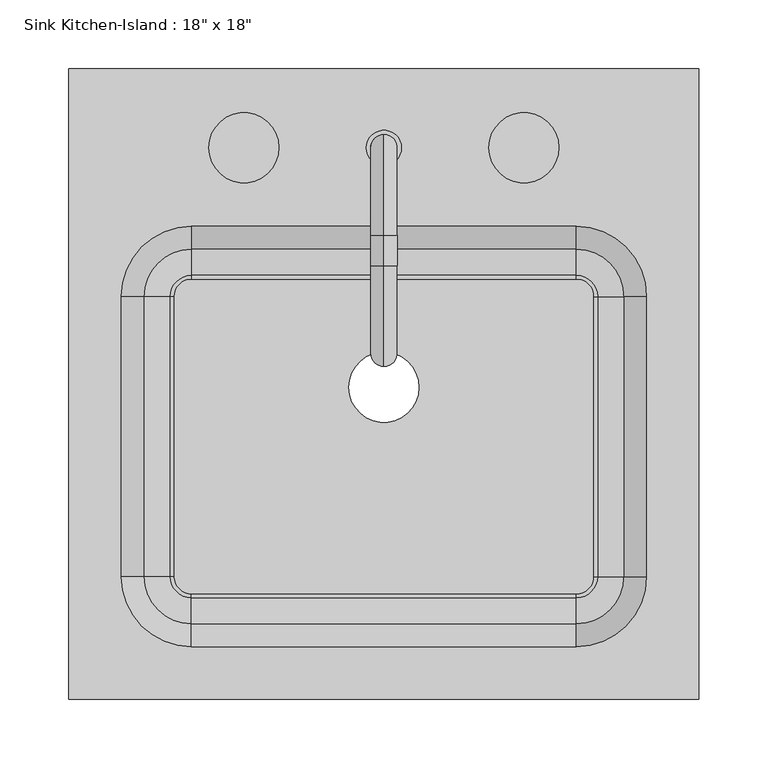
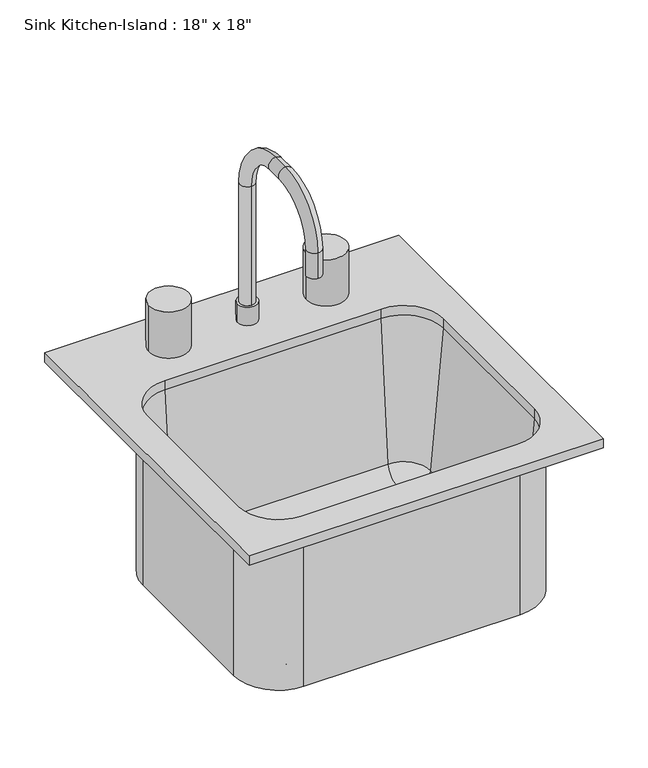
"""IFC4 building model written with IfcOpenShell, lengths in millimetres: flow terminal geometry."""

from ifc_helpers import new_model, si_unit, point, frame, frame_2d, origin, place, context, project, spatial, polyline, circle_curve, ellipse_curve, trimmed, segment, composite_curve, outline, extrude, source, transform, mapped, element, save
from ifc_brep_helpers import plane_surface, cylinder_surface, revolved_surface, advanced_brep


def flow_terminal_871c2e40(model_context):
    return source(origin(), model_context, "Body", "SolidModel", [
        advanced_brep(
        [(244.2892406, 230.9454011, 927.1), (-212.9107594, 230.9454011, 927.1), (-212.9107594, -226.2545989, 927.1), (244.2892406, -226.2545989, 927.1), (155.3892406, 116.6454011, 927.1), (206.1892406, 65.8454011, 927.1), (206.1892406, -137.3545989, 927.1), (155.3892406, -188.1545989, 927.1), (-124.0107594, -188.1545989, 927.1), (-174.8107594, -137.3545989, 927.1), (-174.8107594, 65.8454011, 927.1), (-124.0107594, 116.6454011, 927.1), (244.2892406, 230.9454011, 914.4), (244.2892406, -226.2545989, 914.4), (-212.9107594, -226.2545989, 914.4), (-212.9107594, 230.9454011, 914.4), (212.5392406, 65.8454011, 914.4), (155.3892406, 122.9954011, 914.4), (-124.0107594, 122.9954011, 914.4), (-181.1607594, 65.8454011, 914.4), (-181.1607594, -137.3545989, 914.4), (-124.0107594, -194.5045989, 914.4), (155.3892406, -194.5045989, 914.4), (212.5392406, -137.3545989, 914.4), (155.3892406, 116.6454011, 914.4), (206.1892406, 65.8454011, 914.4), (206.1892406, -137.3545989, 914.4), (155.3892406, -188.1545989, 914.4), (-124.0107594, -188.1545989, 914.4), (-174.8107594, -137.3545989, 914.4), (-174.8107594, 65.8454011, 914.4), (-124.0107594, 116.6454011, 914.4), (212.5392406, 65.8454011, 698.5), (155.3892406, 122.9954011, 698.5), (168.0892406, 65.8454011, 698.5), (155.3892406, 78.5454011, 698.5), (168.0892406, 65.8454011, 708.025), (155.3892406, 78.5454011, 708.025), (170.6776588, 65.8454011, 708.025), (155.3892406, 81.1338193, 708.025), (189.6551678, 65.8454011, 725.4146831), (155.3892406, 100.1113283, 725.4146831), (212.5392406, -137.3545989, 698.5), (168.0892406, -137.3545989, 698.5), (168.0892406, -137.3545989, 708.025), (170.6776588, -137.3545989, 708.025), (189.6551678, -137.3545989, 725.4146831), (155.3892406, -194.5045989, 698.5), (155.3892406, -150.0545989, 698.5), (155.3892406, -150.0545989, 708.025), (155.3892406, -152.6430171, 708.025), (155.3892406, -171.6205261, 725.4146831), (-124.0107594, -194.5045989, 698.5), (-124.0107594, -150.0545989, 698.5), (-124.0107594, -150.0545989, 708.025), (-124.0107594, -152.6430171, 708.025), (-124.0107594, -171.6205261, 725.4146831), (-181.1607594, -137.3545989, 698.5), (-136.7107594, -137.3545989, 698.5), (-136.7107594, -137.3545989, 708.025), (-139.2991776, -137.3545989, 708.025), (-158.2766866, -137.3545989, 725.4146831), (-181.1607594, 65.8454011, 698.5), (-136.7107594, 65.8454011, 698.5), (-136.7107594, 65.8454011, 708.025), (-139.2991776, 65.8454011, 708.025), (-158.2766866, 65.8454011, 725.4146831), (-124.0107594, 122.9954011, 698.5), (-124.0107594, 78.5454011, 698.5), (-124.0107594, 78.5454011, 708.025), (-124.0107594, 81.1338193, 708.025), (-124.0107594, 100.1113283, 725.4146831)],
        [
            (0, 1),
            (1, 2),
            (2, 3),
            (3, 0),
            (4, 5, circle_curve(frame((155.3892406, 65.8454011, 927.1), z_axis=(0.0, 0.0, -1.0), x_axis=(1.0, 0.0, 0.0)), 50.8)),
            (5, 6),
            (6, 7, circle_curve(frame((155.3892406, -137.3545989, 927.1), z_axis=(0.0, 0.0, -1.0), x_axis=(1.0, 0.0, 0.0)), 50.8)),
            (7, 8),
            (8, 9, circle_curve(frame((-124.0107594, -137.3545989, 927.1), z_axis=(0.0, 0.0, -1.0), x_axis=(1.0, 0.0, 0.0)), 50.8)),
            (9, 10),
            (10, 11, circle_curve(frame((-124.0107594, 65.8454011, 927.1), z_axis=(0.0, 0.0, -1.0), x_axis=(1.0, 0.0, 0.0)), 50.8)),
            (11, 4),
            (12, 13),
            (13, 14),
            (14, 15),
            (15, 12),
            (16, 17, circle_curve(frame((155.3892406, 65.8454011, 914.4), z_axis=(0.0, 0.0, 1.0), x_axis=(0.0, 1.0, 0.0)), 57.15)),
            (17, 18),
            (18, 19, circle_curve(frame((-124.0107594, 65.8454011, 914.4), z_axis=(0.0, 0.0, 1.0), x_axis=(-1.0, 0.0, 0.0)), 57.15)),
            (19, 20),
            (20, 21, circle_curve(frame((-124.0107594, -137.3545989, 914.4), z_axis=(0.0, 0.0, 1.0), x_axis=(0.0, -1.0, 0.0)), 57.15)),
            (21, 22),
            (22, 23, circle_curve(frame((155.3892406, -137.3545989, 914.4), z_axis=(0.0, 0.0, 1.0), x_axis=(1.0, 0.0, 0.0)), 57.15)),
            (23, 16),
            (0, 12),
            (15, 1),
            (14, 2),
            (13, 3),
            (4, 24),
            (24, 25, circle_curve(frame((155.3892406, 65.8454011, 914.4), z_axis=(0.0, 0.0, -1.0), x_axis=(1.0, 0.0, 0.0)), 50.8)),
            (25, 5),
            (25, 26),
            (26, 6),
            (26, 27, circle_curve(frame((155.3892406, -137.3545989, 914.4), z_axis=(0.0, 0.0, -1.0), x_axis=(1.0, 0.0, 0.0)), 50.8)),
            (27, 7),
            (27, 28),
            (28, 8),
            (28, 29, circle_curve(frame((-124.0107594, -137.3545989, 914.4), z_axis=(0.0, 0.0, -1.0), x_axis=(1.0, 0.0, 0.0)), 50.8)),
            (29, 9),
            (29, 30),
            (30, 10),
            (30, 31, circle_curve(frame((-124.0107594, 65.8454011, 914.4), z_axis=(0.0, 0.0, -1.0), x_axis=(1.0, 0.0, 0.0)), 50.8)),
            (31, 11),
            (31, 24),
            (32, 33, circle_curve(frame((155.3892406, 65.8454011, 698.5), z_axis=(0.0, 0.0, 1.0), x_axis=(0.0, 1.0, 0.0)), 57.15)),
            (33, 17),
            (16, 32),
            (32, 34),
            (34, 35, circle_curve(frame((155.3892406, 65.8454011, 698.5), z_axis=(0.0, 0.0, 1.0), x_axis=(0.0, 1.0, 0.0)), 12.7)),
            (35, 33),
            (34, 36),
            (36, 37, circle_curve(frame((155.3892406, 65.8454011, 708.025), z_axis=(0.0, 0.0, 1.0), x_axis=(0.0, 1.0, 0.0)), 12.7)),
            (37, 35),
            (36, 38),
            (38, 39, circle_curve(frame((155.3892406, 65.8454011, 708.025), z_axis=(0.0, 0.0, 1.0), x_axis=(0.0, 1.0, 0.0)), 15.2884182)),
            (39, 37),
            (38, 40, circle_curve(frame((170.6776588, 65.8454011, 727.075), z_axis=(0.0, -1.0, 0.0), x_axis=(1.0, 0.0, 0.0)), 19.05)),
            (40, 41, circle_curve(frame((155.3892406, 65.8454011, 725.4146831), z_axis=(0.0, 0.0, 1.0), x_axis=(0.0, 1.0, 0.0)), 34.2659272)),
            (41, 39, circle_curve(frame((155.3892406, 81.1338193, 727.075), z_axis=(-1.0, 0.0, 0.0), x_axis=(0.0, 1.0, 0.0)), 19.05)),
            (40, 25),
            (24, 41),
            (23, 42),
            (42, 32),
            (42, 43),
            (43, 34),
            (43, 44),
            (44, 36),
            (44, 45),
            (45, 38),
            (45, 46, circle_curve(frame((170.6776588, -137.3545989, 727.075), z_axis=(0.0, -1.0, 0.0), x_axis=(1.0, 0.0, 0.0)), 19.05)),
            (46, 40),
            (46, 26),
            (22, 47),
            (47, 42, circle_curve(frame((155.3892406, -137.3545989, 698.5), z_axis=(0.0, 0.0, 1.0), x_axis=(1.0, 0.0, 0.0)), 57.15)),
            (47, 48),
            (48, 43, circle_curve(frame((155.3892406, -137.3545989, 698.5), z_axis=(0.0, 0.0, 1.0), x_axis=(1.0, 0.0, 0.0)), 12.7)),
            (48, 49),
            (49, 44, circle_curve(frame((155.3892406, -137.3545989, 708.025), z_axis=(0.0, 0.0, 1.0), x_axis=(1.0, 0.0, 0.0)), 12.7)),
            (49, 50),
            (50, 45, circle_curve(frame((155.3892406, -137.3545989, 708.025), z_axis=(0.0, 0.0, 1.0), x_axis=(1.0, 0.0, 0.0)), 15.2884182)),
            (50, 51, circle_curve(frame((155.3892406, -152.6430171, 727.075), z_axis=(-1.0, 0.0, 0.0), x_axis=(0.0, -1.0, 0.0)), 19.05)),
            (51, 46, circle_curve(frame((155.3892406, -137.3545989, 725.4146831), z_axis=(0.0, 0.0, 1.0), x_axis=(1.0, 0.0, 0.0)), 34.2659272)),
            (51, 27),
            (21, 52),
            (52, 47),
            (52, 53),
            (53, 48),
            (53, 54),
            (54, 49),
            (54, 55),
            (55, 50),
            (55, 56, circle_curve(frame((-124.0107594, -152.6430171, 727.075), z_axis=(-1.0, 0.0, 0.0), x_axis=(0.0, -1.0, 0.0)), 19.05)),
            (56, 51),
            (56, 28),
            (20, 57),
            (57, 52, circle_curve(frame((-124.0107594, -137.3545989, 698.5), z_axis=(0.0, 0.0, 1.0), x_axis=(0.0, -1.0, 0.0)), 57.15)),
            (57, 58),
            (58, 53, circle_curve(frame((-124.0107594, -137.3545989, 698.5), z_axis=(0.0, 0.0, 1.0), x_axis=(0.0, -1.0, 0.0)), 12.7)),
            (58, 59),
            (59, 54, circle_curve(frame((-124.0107594, -137.3545989, 708.025), z_axis=(0.0, 0.0, 1.0), x_axis=(0.0, -1.0, 0.0)), 12.7)),
            (59, 60),
            (60, 55, circle_curve(frame((-124.0107594, -137.3545989, 708.025), z_axis=(0.0, 0.0, 1.0), x_axis=(0.0, -1.0, 0.0)), 15.2884182)),
            (60, 61, circle_curve(frame((-139.2991776, -137.3545989, 727.075), z_axis=(0.0, 1.0, 0.0), x_axis=(-1.0, 0.0, 0.0)), 19.05)),
            (61, 56, circle_curve(frame((-124.0107594, -137.3545989, 725.4146831), z_axis=(0.0, 0.0, 1.0), x_axis=(0.0, -1.0, 0.0)), 34.2659272)),
            (61, 29),
            (19, 62),
            (62, 57),
            (62, 63),
            (63, 58),
            (63, 64),
            (64, 59),
            (64, 65),
            (65, 60),
            (65, 66, circle_curve(frame((-139.2991776, 65.8454011, 727.075), z_axis=(0.0, 1.0, 0.0), x_axis=(-1.0, 0.0, 0.0)), 19.05)),
            (66, 61),
            (66, 30),
            (18, 67),
            (67, 62, circle_curve(frame((-124.0107594, 65.8454011, 698.5), z_axis=(0.0, 0.0, 1.0), x_axis=(-1.0, 0.0, 0.0)), 57.15)),
            (67, 68),
            (68, 63, circle_curve(frame((-124.0107594, 65.8454011, 698.5), z_axis=(0.0, 0.0, 1.0), x_axis=(-1.0, 0.0, 0.0)), 12.7)),
            (68, 69),
            (69, 64, circle_curve(frame((-124.0107594, 65.8454011, 708.025), z_axis=(0.0, 0.0, 1.0), x_axis=(-1.0, 0.0, 0.0)), 12.7)),
            (69, 70),
            (70, 65, circle_curve(frame((-124.0107594, 65.8454011, 708.025), z_axis=(0.0, 0.0, 1.0), x_axis=(-1.0, 0.0, 0.0)), 15.2884182)),
            (70, 71, circle_curve(frame((-124.0107594, 81.1338193, 727.075), z_axis=(1.0, 0.0, 0.0), x_axis=(0.0, 1.0, 0.0)), 19.05)),
            (71, 66, circle_curve(frame((-124.0107594, 65.8454011, 725.4146831), z_axis=(0.0, 0.0, 1.0), x_axis=(-1.0, 0.0, 0.0)), 34.2659272)),
            (71, 31),
            (33, 67),
            (35, 68),
            (37, 69),
            (39, 70),
            (41, 71),
        ],
        [
            plane_surface(frame((-212.9107594, 230.9454011, 927.1), z_axis=(0.0, 0.0, 1.0), x_axis=(-1.0, 0.0, 0.0))),
            plane_surface(frame((-212.9107594, 230.9454011, 914.4), z_axis=(0.0, 0.0, -1.0), x_axis=(1.0, 0.0, 0.0))),
            plane_surface(frame((244.2892406, 230.9454011, 927.1), z_axis=(0.0, 1.0, 0.0), x_axis=(0.0, 0.0, -1.0))),
            plane_surface(frame((-212.9107594, 230.9454011, 927.1), z_axis=(-1.0, 0.0, 0.0), x_axis=(0.0, 0.0, -1.0))),
            plane_surface(frame((-212.9107594, -226.2545989, 927.1), z_axis=(0.0, -1.0, 0.0), x_axis=(0.0, 0.0, -1.0))),
            plane_surface(frame((244.2892406, -226.2545989, 927.1), z_axis=(1.0, 0.0, 0.0), x_axis=(0.0, 0.0, -1.0))),
            revolved_surface(polyline([(206.1892406, 65.8454011, 914.4), (206.1892406, 65.8454011, 927.1)]), (155.3892406, 65.8454011, 0.0), (0.0, 0.0, -1.0)),
            plane_surface(frame((206.1892406, 65.8454011, 927.1), z_axis=(-1.0, 0.0, 0.0), x_axis=(0.0, 0.0, -1.0))),
            revolved_surface(polyline([(206.1892406, -137.3545989, 914.4), (206.1892406, -137.3545989, 927.1)]), (155.3892406, -137.3545989, 0.0), (0.0, 0.0, -1.0)),
            plane_surface(frame((155.3892406, -188.1545989, 927.1), z_axis=(0.0, 1.0, 0.0), x_axis=(0.0, 0.0, -1.0))),
            revolved_surface(polyline([(-73.2107594, -137.3545989, 914.4), (-73.2107594, -137.3545989, 927.1)]), (-124.0107594, -137.3545989, 0.0), (0.0, 0.0, -1.0)),
            plane_surface(frame((-174.8107594, -137.3545989, 927.1), z_axis=(1.0, 0.0, 0.0), x_axis=(0.0, 0.0, -1.0))),
            revolved_surface(polyline([(-73.2107594, 65.8454011, 914.4), (-73.2107594, 65.8454011, 927.1)]), (-124.0107594, 65.8454011, 0.0), (0.0, 0.0, -1.0)),
            plane_surface(frame((-124.0107594, 116.6454011, 927.1), z_axis=(0.0, -1.0, 0.0), x_axis=(0.0, 0.0, -1.0))),
            cylinder_surface(frame((155.3892406, 65.8454011, 0.0), z_axis=(0.0, 0.0, -1.0), x_axis=(0.0, 1.0, 0.0)), 57.15),
            plane_surface(frame((155.3892406, 65.8454011, 698.5), z_axis=(0.0, 0.0, -1.0), x_axis=(0.0, 1.0, 0.0))),
            revolved_surface(polyline([(155.3892406, 78.5454011, 698.5), (155.3892406, 78.5454011, 708.025)]), (155.3892406, 65.8454011, 0.0), (0.0, 0.0, -1.0)),
            plane_surface(frame((155.3892406, 65.8454011, 708.025), z_axis=(0.0, 0.0, 1.0), x_axis=(0.0, 1.0, 0.0))),
            revolved_surface(trimmed(ellipse_curve(frame((155.3892406, 81.1338193, 727.075), z_axis=(1.0, 0.0, 0.0), x_axis=(0.0, 1.0, 0.0)), 19.05, 19.05), [point((155.3892406, 81.1338193, 708.025))], [point((155.3892406, 100.1113283, 725.4146831))], True, "CARTESIAN"), (155.3892406, 65.8454011, 0.0), (0.0, 0.0, -1.0)),
            revolved_surface(polyline([(155.3892406, 100.1113283, 725.4146831), (155.3892406, 116.6454011, 914.4)]), (155.3892406, 65.8454011, 0.0), (0.0, 0.0, -1.0)),
            plane_surface(frame((212.5392406, 65.8454011, 914.4), z_axis=(1.0, 0.0, 0.0), x_axis=(0.0, -1.0, 0.0))),
            plane_surface(frame((212.5392406, 65.8454011, 698.5), z_axis=(0.0, 0.0, -1.0), x_axis=(0.0, -1.0, 0.0))),
            plane_surface(frame((168.0892406, 65.8454011, 698.5), z_axis=(-1.0, 0.0, 0.0), x_axis=(0.0, -1.0, 0.0))),
            plane_surface(frame((168.0892406, 65.8454011, 708.025), z_axis=(0.0, 0.0, 1.0), x_axis=(0.0, -1.0, 0.0))),
            revolved_surface(polyline([(189.7276588, -137.3545989, 727.075), (189.7276588, 65.8454011, 727.075)]), (170.6776588, 65.8454011, 727.075), (0.0, -1.0, 0.0)),
            plane_surface(frame((189.6551678, 65.8454011, 725.4146831), z_axis=(-0.9961946980917443, 0.0, 0.08715574274767254), x_axis=(0.0, -1.0, 0.0))),
            cylinder_surface(frame((155.3892406, -137.3545989, 0.0), z_axis=(0.0, 0.0, -1.0), x_axis=(1.0, 0.0, 0.0)), 57.15),
            plane_surface(frame((155.3892406, -137.3545989, 698.5), z_axis=(0.0, 0.0, -1.0), x_axis=(1.0, 0.0, 0.0))),
            revolved_surface(polyline([(168.08924059999998, -137.3545989, 698.5), (168.08924059999998, -137.3545989, 708.025)]), (155.3892406, -137.3545989, 0.0), (0.0, 0.0, -1.0)),
            plane_surface(frame((155.3892406, -137.3545989, 708.025), z_axis=(0.0, 0.0, 1.0), x_axis=(1.0, 0.0, 0.0))),
            revolved_surface(trimmed(ellipse_curve(frame((170.6776588, -137.3545989, 727.075), z_axis=(0.0, -1.0, 0.0), x_axis=(1.0, 0.0, 0.0)), 19.05, 19.05), [point((170.6776588, -137.3545989, 708.025))], [point((189.6551678, -137.3545989, 725.4146831))], True, "CARTESIAN"), (155.3892406, -137.3545989, 0.0), (0.0, 0.0, -1.0)),
            revolved_surface(polyline([(189.6551678, -137.3545989, 725.4146831), (206.1892406, -137.3545989, 914.4)]), (155.3892406, -137.3545989, 0.0), (0.0, 0.0, -1.0)),
            plane_surface(frame((155.3892406, -194.5045989, 914.4), z_axis=(0.0, -1.0, 0.0), x_axis=(-1.0, 0.0, 0.0))),
            plane_surface(frame((155.3892406, -194.5045989, 698.5), z_axis=(0.0, 0.0, -1.0), x_axis=(-1.0, 0.0, 0.0))),
            plane_surface(frame((155.3892406, -150.0545989, 698.5), z_axis=(0.0, 1.0, 0.0), x_axis=(-1.0, 0.0, 0.0))),
            plane_surface(frame((155.3892406, -150.0545989, 708.025), z_axis=(0.0, 0.0, 1.0), x_axis=(-1.0, 0.0, 0.0))),
            revolved_surface(polyline([(-124.01075939999998, -171.69301710000002, 727.075), (155.3892406, -171.69301710000002, 727.075)]), (155.3892406, -152.6430171, 727.075), (-1.0, 0.0, 0.0)),
            plane_surface(frame((155.3892406, -171.6205261, 725.4146831), z_axis=(0.0, 0.9961946980917443, 0.08715574274767254), x_axis=(-1.0, 0.0, 0.0))),
            cylinder_surface(frame((-124.0107594, -137.3545989, 0.0), z_axis=(0.0, 0.0, -1.0), x_axis=(0.0, -1.0, 0.0)), 57.15),
            plane_surface(frame((-124.0107594, -137.3545989, 698.5), z_axis=(0.0, 0.0, -1.0), x_axis=(0.0, -1.0, 0.0))),
            revolved_surface(polyline([(-124.0107594, -150.0545989, 698.5), (-124.0107594, -150.0545989, 708.025)]), (-124.0107594, -137.3545989, 0.0), (0.0, 0.0, -1.0)),
            plane_surface(frame((-124.0107594, -137.3545989, 708.025), z_axis=(0.0, 0.0, 1.0), x_axis=(0.0, -1.0, 0.0))),
            revolved_surface(trimmed(ellipse_curve(frame((-124.0107594, -152.6430171, 727.075), z_axis=(-1.0, 0.0, 0.0), x_axis=(0.0, -1.0, 0.0)), 19.05, 19.05), [point((-124.0107594, -152.6430171, 708.025))], [point((-124.0107594, -171.6205261, 725.4146831))], True, "CARTESIAN"), (-124.0107594, -137.3545989, 0.0), (0.0, 0.0, -1.0)),
            revolved_surface(polyline([(-124.0107594, -171.6205261, 725.4146831), (-124.0107594, -188.1545989, 914.4)]), (-124.0107594, -137.3545989, 0.0), (0.0, 0.0, -1.0)),
            plane_surface(frame((-181.1607594, -137.3545989, 914.4), z_axis=(-1.0, 0.0, 0.0), x_axis=(0.0, 1.0, 0.0))),
            plane_surface(frame((-181.1607594, -137.3545989, 698.5), z_axis=(0.0, 0.0, -1.0), x_axis=(0.0, 1.0, 0.0))),
            plane_surface(frame((-136.7107594, -137.3545989, 698.5), z_axis=(1.0, 0.0, 0.0), x_axis=(0.0, 1.0, 0.0))),
            plane_surface(frame((-136.7107594, -137.3545989, 708.025), z_axis=(0.0, 0.0, 1.0), x_axis=(0.0, 1.0, 0.0))),
            revolved_surface(polyline([(-158.34917760000002, 65.8454011, 727.075), (-158.34917760000002, -137.3545989, 727.075)]), (-139.2991776, -137.3545989, 727.075), (0.0, 1.0, 0.0)),
            plane_surface(frame((-158.2766866, -137.3545989, 725.4146831), z_axis=(0.9961946980917443, 0.0, 0.08715574274767254), x_axis=(0.0, 1.0, 0.0))),
            cylinder_surface(frame((-124.0107594, 65.8454011, 0.0), z_axis=(0.0, 0.0, -1.0), x_axis=(-1.0, 0.0, 0.0)), 57.15),
            plane_surface(frame((-124.0107594, 65.8454011, 698.5), z_axis=(0.0, 0.0, -1.0), x_axis=(-1.0, 0.0, 0.0))),
            revolved_surface(polyline([(-136.7107594, 65.8454011, 698.5), (-136.7107594, 65.8454011, 708.025)]), (-124.0107594, 65.8454011, 0.0), (0.0, 0.0, -1.0)),
            plane_surface(frame((-124.0107594, 65.8454011, 708.025), z_axis=(0.0, 0.0, 1.0), x_axis=(-1.0, 0.0, 0.0))),
            revolved_surface(trimmed(ellipse_curve(frame((-139.2991776, 65.8454011, 727.075), z_axis=(0.0, 1.0, 0.0), x_axis=(-1.0, 0.0, 0.0)), 19.05, 19.05), [point((-139.2991776, 65.8454011, 708.025))], [point((-158.2766866, 65.8454011, 725.4146831))], True, "CARTESIAN"), (-124.0107594, 65.8454011, 0.0), (0.0, 0.0, -1.0)),
            revolved_surface(polyline([(-158.2766866, 65.8454011, 725.4146831), (-174.8107594, 65.8454011, 914.4)]), (-124.0107594, 65.8454011, 0.0), (0.0, 0.0, -1.0)),
            plane_surface(frame((-124.0107594, 122.9954011, 914.4), z_axis=(0.0, 1.0, 0.0), x_axis=(1.0, 0.0, 0.0))),
            plane_surface(frame((-124.0107594, 122.9954011, 698.5), z_axis=(0.0, 0.0, -1.0), x_axis=(1.0, 0.0, 0.0))),
            plane_surface(frame((-124.0107594, 78.5454011, 698.5), z_axis=(0.0, -1.0, 0.0), x_axis=(1.0, 0.0, 0.0))),
            plane_surface(frame((-124.0107594, 78.5454011, 708.025), z_axis=(0.0, 0.0, 1.0), x_axis=(1.0, 0.0, 0.0))),
            revolved_surface(polyline([(155.3892406, 100.1838193, 727.075), (-124.0107594, 100.1838193, 727.075)]), (-124.0107594, 81.1338193, 727.075), (1.0, 0.0, 0.0)),
            plane_surface(frame((-124.0107594, 100.1113283, 725.4146831), z_axis=(0.0, -0.9961946980917443, 0.08715574274767254), x_axis=(1.0, 0.0, 0.0))),
        ],
        [
            (0, [[1, 2, 3, 4], [5, 6, 7, 8, 9, 10, 11, 12]]),
            (1, [[13, 14, 15, 16], [17, 18, 19, 20, 21, 22, 23, 24]]),
            (2, [[-1, 25, -16, 26]]),
            (3, [[-2, -26, -15, 27]]),
            (4, [[-3, -27, -14, 28]]),
            (5, [[-4, -28, -13, -25]]),
            (6, [[-5, 29, 30, 31]]),
            (7, [[-6, -31, 32, 33]]),
            (8, [[-7, -33, 34, 35]]),
            (9, [[-8, -35, 36, 37]]),
            (10, [[-9, -37, 38, 39]]),
            (11, [[-10, -39, 40, 41]]),
            (12, [[-11, -41, 42, 43]]),
            (13, [[-12, -43, 44, -29]]),
            (14, [[45, 46, -17, 47]]),
            (15, [[-45, 48, 49, 50]]),
            (16, [[-49, 51, 52, 53]]),
            (17, [[-52, 54, 55, 56]]),
            (18, [[-55, 57, 58, 59]]),
            (19, [[-58, 60, -30, 61]]),
            (20, [[-47, -24, 62, 63]]),
            (21, [[-48, -63, 64, 65]]),
            (22, [[-51, -65, 66, 67]]),
            (23, [[-54, -67, 68, 69]]),
            (24, [[-57, -69, 70, 71]]),
            (25, [[-60, -71, 72, -32]]),
            (26, [[-62, -23, 73, 74]]),
            (27, [[-64, -74, 75, 76]]),
            (28, [[-66, -76, 77, 78]]),
            (29, [[-68, -78, 79, 80]]),
            (30, [[-70, -80, 81, 82]]),
            (31, [[-72, -82, 83, -34]]),
            (32, [[-73, -22, 84, 85]]),
            (33, [[-75, -85, 86, 87]]),
            (34, [[-77, -87, 88, 89]]),
            (35, [[-79, -89, 90, 91]]),
            (36, [[-81, -91, 92, 93]]),
            (37, [[-83, -93, 94, -36]]),
            (38, [[-84, -21, 95, 96]]),
            (39, [[-86, -96, 97, 98]]),
            (40, [[-88, -98, 99, 100]]),
            (41, [[-90, -100, 101, 102]]),
            (42, [[-92, -102, 103, 104]]),
            (43, [[-94, -104, 105, -38]]),
            (44, [[-95, -20, 106, 107]]),
            (45, [[-97, -107, 108, 109]]),
            (46, [[-99, -109, 110, 111]]),
            (47, [[-101, -111, 112, 113]]),
            (48, [[-103, -113, 114, 115]]),
            (49, [[-105, -115, 116, -40]]),
            (50, [[-106, -19, 117, 118]]),
            (51, [[-108, -118, 119, 120]]),
            (52, [[-110, -120, 121, 122]]),
            (53, [[-112, -122, 123, 124]]),
            (54, [[-114, -124, 125, 126]]),
            (55, [[-116, -126, 127, -42]]),
            (56, [[-46, 128, -117, -18]]),
            (57, [[-50, 129, -119, -128]]),
            (58, [[-53, 130, -121, -129]]),
            (59, [[-56, 131, -123, -130]]),
            (60, [[-59, 132, -125, -131]]),
            (61, [[-61, -44, -127, -132]]),
        ],
    ),
        advanced_brep(
        [(2.9892406, 173.7954011, 927.1), (28.3892406, 173.7954011, 927.1), (15.6892406, 183.3204011, 1114.425), (15.6892406, 164.2704011, 1114.425), (15.6892406, 164.2704011, 952.5), (15.6892406, 183.3204011, 952.5), (15.6892406, 110.2954011, 1187.45), (15.6892406, 110.2954011, 1168.4), (15.6892406, 88.0704011, 1187.45), (15.6892406, 88.0704011, 1168.4), (15.6892406, 15.0454011, 1114.425), (15.6892406, 34.0954011, 1114.425), (15.6892406, 15.0454011, 1079.5), (15.6892406, 34.0954011, 1079.5), (2.9892406, 173.7954011, 952.5), (28.3892406, 173.7954011, 952.5)],
        [
            (0, 1, circle_curve(frame((15.6892406, 173.7954011, 927.1), z_axis=(0.0, 0.0, -1.0), x_axis=(1.0, 0.0, 0.0)), 12.7)),
            (1, 0, circle_curve(frame((15.6892406, 173.7954011, 927.1), z_axis=(0.0, 0.0, -1.0), x_axis=(1.0, 0.0, 0.0)), 12.7)),
            (2, 3, circle_curve(frame((15.6892406, 173.7954011, 1114.425), z_axis=(0.0, 0.0, -1.0), x_axis=(0.0, -1.0, 0.0)), 9.525)),
            (3, 4),
            (4, 5, circle_curve(frame((15.6892406, 173.7954011, 952.5), z_axis=(0.0, 0.0, 1.0), x_axis=(0.0, -1.0, 0.0)), 9.525)),
            (5, 2),
            (3, 2, circle_curve(frame((15.6892406, 173.7954011, 1114.425), z_axis=(0.0, 0.0, -1.0), x_axis=(0.0, -1.0, 0.0)), 9.525)),
            (5, 4, circle_curve(frame((15.6892406, 173.7954011, 952.5), z_axis=(0.0, 0.0, 1.0), x_axis=(0.0, -1.0, 0.0)), 9.525)),
            (2, 6, circle_curve(frame((15.6892406, 110.2954011, 1114.425), z_axis=(1.0, 0.0, 0.0), x_axis=(0.0, 1.0, 0.0)), 73.025)),
            (6, 7, circle_curve(frame((15.6892406, 110.2954011, 1177.925), z_axis=(0.0, 1.0, 0.0), x_axis=(0.0, 0.0, -1.0)), 9.525)),
            (7, 3, circle_curve(frame((15.6892406, 110.2954011, 1114.425), z_axis=(-1.0, 0.0, 0.0), x_axis=(0.0, 1.0, 0.0)), 53.975)),
            (7, 6, circle_curve(frame((15.6892406, 110.2954011, 1177.925), z_axis=(0.0, 1.0, 0.0), x_axis=(0.0, 0.0, -1.0)), 9.525)),
            (6, 8),
            (8, 9, circle_curve(frame((15.6892406, 88.0704011, 1177.925), z_axis=(0.0, 1.0, 0.0), x_axis=(0.0, 0.0, -1.0)), 9.525)),
            (9, 7),
            (9, 8, circle_curve(frame((15.6892406, 88.0704011, 1177.925), z_axis=(0.0, 1.0, 0.0), x_axis=(0.0, 0.0, -1.0)), 9.525)),
            (8, 10, circle_curve(frame((15.6892406, 88.0704011, 1114.425), z_axis=(1.0, 0.0, 0.0), x_axis=(0.0, 0.0, 1.0)), 73.025)),
            (10, 11, circle_curve(frame((15.6892406, 24.5704011, 1114.425), z_axis=(0.0, 0.0, 1.0), x_axis=(0.0, 1.0, 0.0)), 9.525)),
            (11, 9, circle_curve(frame((15.6892406, 88.0704011, 1114.425), z_axis=(-1.0, 0.0, 0.0), x_axis=(0.0, 0.0, 1.0)), 53.975)),
            (11, 10, circle_curve(frame((15.6892406, 24.5704011, 1114.425), z_axis=(0.0, 0.0, 1.0), x_axis=(0.0, 1.0, 0.0)), 9.525)),
            (12, 13, circle_curve(frame((15.6892406, 24.5704011, 1079.5), z_axis=(0.0, 0.0, -1.0), x_axis=(0.0, 1.0, 0.0)), 9.525)),
            (13, 12, circle_curve(frame((15.6892406, 24.5704011, 1079.5), z_axis=(0.0, 0.0, -1.0), x_axis=(0.0, 1.0, 0.0)), 9.525)),
            (10, 12),
            (13, 11),
            (14, 15, circle_curve(frame((15.6892406, 173.7954011, 952.5), z_axis=(0.0, 0.0, 1.0), x_axis=(1.0, 0.0, 0.0)), 12.7)),
            (15, 14, circle_curve(frame((15.6892406, 173.7954011, 952.5), z_axis=(0.0, 0.0, 1.0), x_axis=(1.0, 0.0, 0.0)), 12.7)),
            (14, 0),
            (1, 15),
        ],
        [
            plane_surface(frame((15.6892406, 164.2704011, 927.1), z_axis=(0.0, 0.0, -1.0), x_axis=(1.0, 0.0, 0.0))),
            cylinder_surface(frame((15.6892406, 173.7954011, 927.1), z_axis=(0.0, 0.0, -1.0), x_axis=(0.0, -1.0, 0.0)), 9.525),
            revolved_surface(trimmed(ellipse_curve(frame((15.6892406, 173.7954011, 1114.425), z_axis=(0.0, 0.0, -1.0), x_axis=(0.0, -1.0, 0.0)), 9.525, 9.525), [point((15.6892406, 183.3204011, 1114.425))], [point((15.6892406, 164.2704011, 1114.425))], True, "CARTESIAN"), (15.6892406, 110.2954011, 1114.425), (1.0, 0.0, 0.0)),
            revolved_surface(trimmed(ellipse_curve(frame((15.6892406, 173.7954011, 1114.425), z_axis=(0.0, 0.0, -1.0), x_axis=(0.0, -1.0, 0.0)), 9.525, 9.525), [point((15.6892406, 164.2704011, 1114.425))], [point((15.6892406, 183.3204011, 1114.425))], True, "CARTESIAN"), (15.6892406, 110.2954011, 1114.425), (1.0, 0.0, 0.0)),
            cylinder_surface(frame((15.6892406, 110.2954011, 1177.925), z_axis=(0.0, 1.0, 0.0), x_axis=(0.0, 0.0, -1.0)), 9.525),
            revolved_surface(trimmed(ellipse_curve(frame((15.6892406, 88.0704011, 1177.925), z_axis=(0.0, 1.0, 0.0), x_axis=(0.0, 0.0, -1.0)), 9.525, 9.525), [point((15.6892406, 88.0704011, 1187.45))], [point((15.6892406, 88.0704011, 1168.4))], True, "CARTESIAN"), (15.6892406, 88.0704011, 1114.425), (1.0, 0.0, 0.0)),
            revolved_surface(trimmed(ellipse_curve(frame((15.6892406, 88.0704011, 1177.925), z_axis=(0.0, 1.0, 0.0), x_axis=(0.0, 0.0, -1.0)), 9.525, 9.525), [point((15.6892406, 88.0704011, 1168.4))], [point((15.6892406, 88.0704011, 1187.45))], True, "CARTESIAN"), (15.6892406, 88.0704011, 1114.425), (1.0, 0.0, 0.0)),
            plane_surface(frame((15.6892406, 15.0454011, 1079.5), z_axis=(0.0, 0.0, -1.0), x_axis=(-1.0, 0.0, 0.0))),
            cylinder_surface(frame((15.6892406, 24.5704011, 1114.425), z_axis=(0.0, 0.0, 1.0), x_axis=(0.0, 1.0, 0.0)), 9.525),
            plane_surface(frame((28.3892406, 173.7954011, 952.5), z_axis=(0.0, 0.0, 1.0), x_axis=(0.0, 1.0, 0.0))),
            cylinder_surface(frame((15.6892406, 173.7954011, 927.1), z_axis=(0.0, 0.0, 1.0), x_axis=(1.0, 0.0, 0.0)), 12.7),
        ],
        [
            (0, [[1, 2]]),
            (1, [[3, 4, 5, 6]]),
            (1, [[7, -6, 8, -4]]),
            (2, [[-3, 9, 10, 11]]),
            (3, [[-7, -11, 12, -9]]),
            (4, [[-10, 13, 14, 15]]),
            (4, [[-12, -15, 16, -13]]),
            (5, [[-14, 17, 18, 19]]),
            (6, [[-16, -19, 20, -17]]),
            (7, [[21, 22]]),
            (8, [[-18, 23, -22, 24]]),
            (8, [[-20, -24, -21, -23]]),
            (9, [[25, 26], [-5, -8]]),
            (10, [[-25, 27, -2, 28]]),
            (10, [[-26, -28, -1, -27]]),
        ],
    ),
        extrude(outline(composite_curve([segment(trimmed(circle_curve(frame_2d((-85.9107594, 173.7954011)), 25.4), [point((-111.3107594, 173.7954011))], [point((-60.5107594, 173.7954011))], False, "CARTESIAN"), True, "CONTINUOUS"), segment(trimmed(circle_curve(frame_2d((-85.9107594, 173.7954011)), 25.4), [point((-60.5107594, 173.7954011))], [point((-111.3107594, 173.7954011))], False, "CARTESIAN"), True, "CONTINUOUS")], self_intersect=False)), frame((0.0, 0.0, 927.1), z_axis=(0.0, 0.0, 1.0), x_axis=(1.0, 0.0, 0.0)), (0.0, 0.0, 1.0), 63.5),
        extrude(outline(composite_curve([segment(trimmed(circle_curve(frame_2d((117.2892406, 173.7954011)), 25.4), [point((91.8892406, 173.7954011))], [point((142.6892406, 173.7954011))], False, "CARTESIAN"), True, "CONTINUOUS"), segment(trimmed(circle_curve(frame_2d((117.2892406, 173.7954011)), 25.4), [point((142.6892406, 173.7954011))], [point((91.8892406, 173.7954011))], False, "CARTESIAN"), True, "CONTINUOUS")], self_intersect=False)), frame((0.0, 0.0, 927.1), z_axis=(0.0, 0.0, 1.0), x_axis=(1.0, 0.0, 0.0)), (0.0, 0.0, 1.0), 63.5),
        extrude(outline(composite_curve([segment(trimmed(circle_curve(frame_2d((155.3892406, 65.8454011)), 12.7), [point((155.3892406, 78.5454011))], [point((168.0892406, 65.8454011))], False, "CARTESIAN"), True, "CONTINUOUS"), segment(polyline([(168.0892406, 65.8454011), (168.0892406, -137.3545989)]), True, "CONTINUOUS"), segment(trimmed(circle_curve(frame_2d((155.3892406, -137.3545989)), 12.7), [point((168.0892406, -137.3545989))], [point((155.3892406, -150.0545989))], False, "CARTESIAN"), True, "CONTINUOUS"), segment(polyline([(155.3892406, -150.0545989), (-124.0107594, -150.0545989)]), True, "CONTINUOUS"), segment(trimmed(circle_curve(frame_2d((-124.0107594, -137.3545989)), 12.7), [point((-124.0107594, -150.0545989))], [point((-136.7107594, -137.3545989))], False, "CARTESIAN"), True, "CONTINUOUS"), segment(polyline([(-136.7107594, -137.3545989), (-136.7107594, 65.8454011)]), True, "CONTINUOUS"), segment(trimmed(circle_curve(frame_2d((-124.0107594, 65.8454011)), 12.7), [point((-136.7107594, 65.8454011))], [point((-124.0107594, 78.5454011))], False, "CARTESIAN"), True, "CONTINUOUS"), segment(polyline([(-124.0107594, 78.5454011), (155.3892406, 78.5454011)]), True, "CONTINUOUS")], self_intersect=False), holes=[composite_curve([segment(trimmed(circle_curve(frame_2d((15.6892406, 0.0)), 25.4), [point((-9.7107594, 0.0))], [point((41.0892406, 0.0))], True, "CARTESIAN"), True, "CONTINUOUS"), segment(trimmed(circle_curve(frame_2d((15.6892406, 0.0)), 25.4), [point((41.0892406, 0.0))], [point((-9.7107594, 0.0))], True, "CARTESIAN"), True, "CONTINUOUS")], self_intersect=False)]), frame((0.0, 0.0, 698.5), z_axis=(0.0, 0.0, 1.0), x_axis=(1.0, 0.0, 0.0)), (0.0, 0.0, 1.0), 9.525),
    ])


if __name__ == "__main__":
    model = new_model("IFC4")
    model_context = context("Model", 3, world=origin())
    ifc_project = project(units=[si_unit("LENGTHUNIT", "METRE", prefix="MILLI")], contexts=[model_context])
    site = spatial("IfcSite", under=ifc_project)
    building = spatial("IfcBuilding", under=site)
    placement = place(None, origin())
    flow_terminal_shape = flow_terminal_871c2e40(model_context)
    element("IfcFlowTerminal", 1, ObjectType="Sink Kitchen-Island : 18\" x 18\"", at=placement, inside=building, context=model_context, shape_type="MappedRepresentation", body=[
        mapped(flow_terminal_shape, transform((0.0, 0.0, 0.0), x_axis=(1.0, 0.0, 0.0), y_axis=(0.0, 1.0, 0.0), z_axis=(0.0, 0.0, 1.0))),
    ])
    save(model, "model.ifc")

# Revit data of these elements
# Type "Sink Kitchen-Island : 18\" x 18\""
#   Assembly Code = "D2010410"
#   Counter Height = 3' - 0"
#   Depth = 1' - 6"
#   Width = 1' - 6"
#   Faucet Material = Steel, Polished
#   Sink Material = Steel, Polished
#   Default Elevation = 0
# Element 1 (IfcFlowTerminal, "Sink Kitchen-Island : 18\" x 18\"")
#   Materials on its faces: "Steel, Polished"
# Materials
#   "Steel, Polished": class "Metal", colour RGB 57 57 57, transparency 0, Description = "Polished steel", Cost = 0
